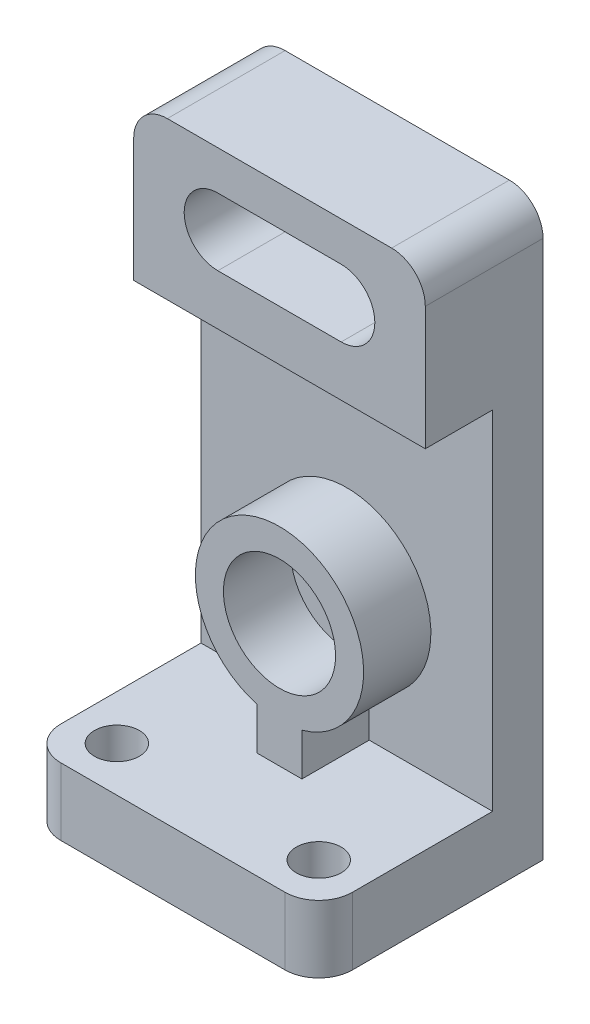
ISO-10303-21;
HEADER;
FILE_DESCRIPTION(('STEP AP214'),'2;1');
FILE_NAME('part.step','',(''),(''),'','','');
FILE_SCHEMA(('AUTOMOTIVE_DESIGN { 1 0 10303 214 1 1 1 1 }'));
ENDSEC;
DATA;
#1=APPLICATION_CONTEXT('core data for automotive mechanical design processes');
#2=APPLICATION_PROTOCOL_DEFINITION('international standard','automotive_design',2000,#1);
#3=PRODUCT_CONTEXT('',#1,'mechanical');
#4=PRODUCT('Part','Part','',(#3));
#5=PRODUCT_RELATED_PRODUCT_CATEGORY('part','',(#4));
#6=PRODUCT_DEFINITION_FORMATION('','',#4);
#7=PRODUCT_DEFINITION_CONTEXT('part definition',#1,'design');
#8=PRODUCT_DEFINITION('design','',#6,#7);
#9=PRODUCT_DEFINITION_SHAPE('','',#8);
#10=(LENGTH_UNIT() NAMED_UNIT(*) SI_UNIT(.MILLI.,.METRE.));
#11=(NAMED_UNIT(*) PLANE_ANGLE_UNIT() SI_UNIT($,.RADIAN.));
#12=(NAMED_UNIT(*) SI_UNIT($,.STERADIAN.) SOLID_ANGLE_UNIT());
#13=UNCERTAINTY_MEASURE_WITH_UNIT(LENGTH_MEASURE(1.E-05),#10,'distance_accuracy_value','');
#14=(GEOMETRIC_REPRESENTATION_CONTEXT(3) GLOBAL_UNCERTAINTY_ASSIGNED_CONTEXT((#13)) GLOBAL_UNIT_ASSIGNED_CONTEXT((#10,
#11,#12)) REPRESENTATION_CONTEXT('',''));
#15=CARTESIAN_POINT('',(0.,0.,0.));
#16=DIRECTION('',(0.,0.,1.));
#17=DIRECTION('',(1.,0.,0.));
#18=AXIS2_PLACEMENT_3D('',#15,#16,#17);
#19=CARTESIAN_POINT('',(46.,96.,9.));
#20=DIRECTION('',(0.,0.,1.));
#21=DIRECTION('',(1.,0.,0.));
#22=AXIS2_PLACEMENT_3D('',#19,#20,#21);
#23=PLANE('',#22);
#24=DIRECTION('',(1.,0.,0.));
#25=VECTOR('',#24,1.);
#26=CARTESIAN_POINT('',(46.,12.,9.));
#27=LINE('',#26,#25);
#28=CARTESIAN_POINT('',(0.,12.,9.));
#29=VERTEX_POINT('',#28);
#30=CARTESIAN_POINT('',(22.,12.,9.));
#31=VERTEX_POINT('',#30);
#32=EDGE_CURVE('E259',#29,#31,#27,.T.);
#33=ORIENTED_EDGE('',*,*,#32,.T.);
#34=DIRECTION('',(0.,-1.,0.));
#35=VECTOR('',#34,1.);
#36=CARTESIAN_POINT('',(22.,12.,9.));
#37=LINE('',#36,#35);
#38=CARTESIAN_POINT('',(22.,19.543167705199,9.));
#39=VERTEX_POINT('',#38);
#40=EDGE_CURVE('E392',#39,#31,#37,.T.);
#41=ORIENTED_EDGE('',*,*,#40,.F.);
#42=CARTESIAN_POINT('',(26.,34.,9.));
#43=DIRECTION('',(0.,0.,1.));
#44=DIRECTION('',(1.,0.,0.));
#45=AXIS2_PLACEMENT_3D('',#42,#43,#44);
#46=CIRCLE('',#45,15.);
#47=CARTESIAN_POINT('',(30.,19.543167705199,9.));
#48=VERTEX_POINT('',#47);
#49=EDGE_CURVE('E203',#48,#39,#46,.T.);
#50=ORIENTED_EDGE('',*,*,#49,.F.);
#51=DIRECTION('',(0.,1.,0.));
#52=VECTOR('',#51,1.);
#53=CARTESIAN_POINT('',(30.,19.543167705199,9.));
#54=LINE('',#53,#52);
#55=CARTESIAN_POINT('',(30.,12.,9.));
#56=VERTEX_POINT('',#55);
#57=EDGE_CURVE('E202',#56,#48,#54,.T.);
#58=ORIENTED_EDGE('',*,*,#57,.F.);
#59=CARTESIAN_POINT('',(52.,12.,9.));
#60=VERTEX_POINT('',#59);
#61=EDGE_CURVE('E252',#56,#60,#27,.T.);
#62=ORIENTED_EDGE('',*,*,#61,.T.);
#63=DIRECTION('',(0.,1.,0.));
#64=VECTOR('',#63,1.);
#65=CARTESIAN_POINT('',(52.,0.,9.));
#66=LINE('',#65,#64);
#67=CARTESIAN_POINT('',(52.,74.,9.));
#68=VERTEX_POINT('',#67);
#69=EDGE_CURVE('E319',#60,#68,#66,.T.);
#70=ORIENTED_EDGE('',*,*,#69,.T.);
#71=DIRECTION('',(-1.,0.,0.));
#72=VECTOR('',#71,1.);
#73=CARTESIAN_POINT('',(0.,74.,9.));
#74=LINE('',#73,#72);
#75=CARTESIAN_POINT('',(0.,74.,9.));
#76=VERTEX_POINT('',#75);
#77=EDGE_CURVE('E289',#68,#76,#74,.T.);
#78=ORIENTED_EDGE('',*,*,#77,.T.);
#79=DIRECTION('',(0.,-1.,0.));
#80=VECTOR('',#79,1.);
#81=CARTESIAN_POINT('',(0.,96.,9.));
#82=LINE('',#81,#80);
#83=EDGE_CURVE('E67',#76,#29,#82,.T.);
#84=ORIENTED_EDGE('',*,*,#83,.T.);
#85=EDGE_LOOP('',(#33,#41,#50,#58,#62,#70,#78,#84));
#86=FACE_BOUND('',#85,.T.);
#87=ADVANCED_FACE('F50',(#86),#23,.T.);
#88=CARTESIAN_POINT('',(46.,12.,34.));
#89=DIRECTION('',(0.,-1.,0.));
#90=DIRECTION('',(0.,0.,-1.));
#91=AXIS2_PLACEMENT_3D('',#88,#89,#90);
#92=PLANE('',#91);
#93=CARTESIAN_POINT('',(44.,12.,32.));
#94=DIRECTION('',(0.,1.,0.));
#95=DIRECTION('',(0.,0.,1.));
#96=AXIS2_PLACEMENT_3D('',#93,#94,#95);
#97=CIRCLE('',#96,4.);
#98=CARTESIAN_POINT('',(44.,12.,36.));
#99=VERTEX_POINT('',#98);
#100=EDGE_CURVE('E210',#99,#99,#97,.T.);
#101=ORIENTED_EDGE('',*,*,#100,.F.);
#102=EDGE_LOOP('',(#101));
#103=FACE_BOUND('',#102,.T.);
#104=CARTESIAN_POINT('',(8.,12.,32.));
#105=DIRECTION('',(0.,1.,0.));
#106=DIRECTION('',(0.,0.,1.));
#107=AXIS2_PLACEMENT_3D('',#104,#105,#106);
#108=CIRCLE('',#107,4.);
#109=CARTESIAN_POINT('',(8.,12.,36.));
#110=VERTEX_POINT('',#109);
#111=EDGE_CURVE('E217',#110,#110,#108,.T.);
#112=ORIENTED_EDGE('',*,*,#111,.F.);
#113=EDGE_LOOP('',(#112));
#114=FACE_BOUND('',#113,.T.);
#115=DIRECTION('',(0.,0.,-1.));
#116=VECTOR('',#115,1.);
#117=CARTESIAN_POINT('',(22.,12.,21.));
#118=LINE('',#117,#116);
#119=CARTESIAN_POINT('',(22.,12.,21.));
#120=VERTEX_POINT('',#119);
#121=EDGE_CURVE('E65',#120,#31,#118,.T.);
#122=ORIENTED_EDGE('',*,*,#121,.T.);
#123=ORIENTED_EDGE('',*,*,#32,.F.);
#124=DIRECTION('',(0.,0.,-1.));
#125=VECTOR('',#124,1.);
#126=CARTESIAN_POINT('',(0.,12.,9.));
#127=LINE('',#126,#125);
#128=CARTESIAN_POINT('',(0.,12.,34.));
#129=VERTEX_POINT('',#128);
#130=EDGE_CURVE('E223',#129,#29,#127,.T.);
#131=ORIENTED_EDGE('',*,*,#130,.F.);
#132=CARTESIAN_POINT('',(6.,12.,34.));
#133=DIRECTION('',(0.,-1.,0.));
#134=DIRECTION('',(0.,0.,-1.));
#135=AXIS2_PLACEMENT_3D('',#132,#133,#134);
#136=CIRCLE('',#135,6.);
#137=CARTESIAN_POINT('',(6.,12.,40.));
#138=VERTEX_POINT('',#137);
#139=EDGE_CURVE('E240',#138,#129,#136,.T.);
#140=ORIENTED_EDGE('',*,*,#139,.F.);
#141=DIRECTION('',(-1.,0.,0.));
#142=VECTOR('',#141,1.);
#143=CARTESIAN_POINT('',(6.,12.,40.));
#144=LINE('',#143,#142);
#145=CARTESIAN_POINT('',(46.,12.,40.));
#146=VERTEX_POINT('',#145);
#147=EDGE_CURVE('E234',#146,#138,#144,.T.);
#148=ORIENTED_EDGE('',*,*,#147,.F.);
#149=CARTESIAN_POINT('',(46.,12.,34.));
#150=DIRECTION('',(0.,-1.,0.));
#151=DIRECTION('',(0.,0.,-1.));
#152=AXIS2_PLACEMENT_3D('',#149,#150,#151);
#153=CIRCLE('',#152,6.);
#154=CARTESIAN_POINT('',(52.,12.,34.));
#155=VERTEX_POINT('',#154);
#156=EDGE_CURVE('E233',#155,#146,#153,.T.);
#157=ORIENTED_EDGE('',*,*,#156,.F.);
#158=DIRECTION('',(0.,0.,1.));
#159=VECTOR('',#158,1.);
#160=CARTESIAN_POINT('',(52.,12.,0.));
#161=LINE('',#160,#159);
#162=EDGE_CURVE('E226',#60,#155,#161,.T.);
#163=ORIENTED_EDGE('',*,*,#162,.F.);
#164=ORIENTED_EDGE('',*,*,#61,.F.);
#165=DIRECTION('',(0.,0.,-1.));
#166=VECTOR('',#165,1.);
#167=CARTESIAN_POINT('',(30.,12.,21.));
#168=LINE('',#167,#166);
#169=CARTESIAN_POINT('',(30.,12.,21.));
#170=VERTEX_POINT('',#169);
#171=EDGE_CURVE('E215',#170,#56,#168,.T.);
#172=ORIENTED_EDGE('',*,*,#171,.F.);
#173=DIRECTION('',(1.,0.,0.));
#174=VECTOR('',#173,1.);
#175=CARTESIAN_POINT('',(30.,12.,21.));
#176=LINE('',#175,#174);
#177=EDGE_CURVE('E192',#120,#170,#176,.T.);
#178=ORIENTED_EDGE('',*,*,#177,.F.);
#179=EDGE_LOOP('',(#122,#123,#131,#140,#148,#157,#163,#164,#172,#178));
#180=FACE_BOUND('',#179,.T.);
#181=ADVANCED_FACE('F382',(#103,#114,#180),#92,.F.);
#182=CARTESIAN_POINT('',(0.,96.,9.));
#183=DIRECTION('',(1.,0.,0.));
#184=DIRECTION('',(0.,0.,-1.));
#185=AXIS2_PLACEMENT_3D('',#182,#183,#184);
#186=PLANE('',#185);
#187=DIRECTION('',(0.,0.,-1.));
#188=VECTOR('',#187,1.);
#189=CARTESIAN_POINT('',(0.,0.,9.));
#190=LINE('',#189,#188);
#191=CARTESIAN_POINT('',(0.,0.,34.));
#192=VERTEX_POINT('',#191);
#193=CARTESIAN_POINT('',(0.,0.,0.));
#194=VERTEX_POINT('',#193);
#195=EDGE_CURVE('E11',#192,#194,#190,.T.);
#196=ORIENTED_EDGE('',*,*,#195,.F.);
#197=DIRECTION('',(0.,-1.,0.));
#198=VECTOR('',#197,1.);
#199=CARTESIAN_POINT('',(0.,12.,34.));
#200=LINE('',#199,#198);
#201=EDGE_CURVE('E247',#129,#192,#200,.T.);
#202=ORIENTED_EDGE('',*,*,#201,.F.);
#203=ORIENTED_EDGE('',*,*,#130,.T.);
#204=ORIENTED_EDGE('',*,*,#83,.F.);
#205=DIRECTION('',(0.,0.,-1.));
#206=VECTOR('',#205,1.);
#207=CARTESIAN_POINT('',(0.,74.,21.));
#208=LINE('',#207,#206);
#209=CARTESIAN_POINT('',(0.,74.,21.));
#210=VERTEX_POINT('',#209);
#211=EDGE_CURVE('E309',#210,#76,#208,.T.);
#212=ORIENTED_EDGE('',*,*,#211,.F.);
#213=DIRECTION('',(0.,-1.,0.));
#214=VECTOR('',#213,1.);
#215=CARTESIAN_POINT('',(0.,0.,21.));
#216=LINE('',#215,#214);
#217=CARTESIAN_POINT('',(0.,96.,21.));
#218=VERTEX_POINT('',#217);
#219=EDGE_CURVE('E308',#218,#210,#216,.T.);
#220=ORIENTED_EDGE('',*,*,#219,.F.);
#221=DIRECTION('',(0.,0.,-1.));
#222=VECTOR('',#221,1.);
#223=CARTESIAN_POINT('',(0.,96.,9.));
#224=LINE('',#223,#222);
#225=CARTESIAN_POINT('',(0.,96.,0.));
#226=VERTEX_POINT('',#225);
#227=EDGE_CURVE('E322',#218,#226,#224,.T.);
#228=ORIENTED_EDGE('',*,*,#227,.T.);
#229=DIRECTION('',(0.,-1.,0.));
#230=VECTOR('',#229,1.);
#231=CARTESIAN_POINT('',(0.,96.,0.));
#232=LINE('',#231,#230);
#233=EDGE_CURVE('E317',#226,#194,#232,.T.);
#234=ORIENTED_EDGE('',*,*,#233,.T.);
#235=EDGE_LOOP('',(#196,#202,#203,#204,#212,#220,#228,#234));
#236=FACE_BOUND('',#235,.T.);
#237=ADVANCED_FACE('F47',(#236),#186,.F.);
#238=CARTESIAN_POINT('',(0.,0.,9.));
#239=DIRECTION('',(0.,1.,0.));
#240=DIRECTION('',(0.,0.,1.));
#241=AXIS2_PLACEMENT_3D('',#238,#239,#240);
#242=PLANE('',#241);
#243=CARTESIAN_POINT('',(8.,0.,32.));
#244=DIRECTION('',(0.,1.,0.));
#245=DIRECTION('',(0.,0.,1.));
#246=AXIS2_PLACEMENT_3D('',#243,#244,#245);
#247=CIRCLE('',#246,4.);
#248=CARTESIAN_POINT('',(8.,0.,36.));
#249=VERTEX_POINT('',#248);
#250=EDGE_CURVE('E218',#249,#249,#247,.T.);
#251=ORIENTED_EDGE('',*,*,#250,.T.);
#252=EDGE_LOOP('',(#251));
#253=FACE_BOUND('',#252,.T.);
#254=CARTESIAN_POINT('',(44.,0.,32.));
#255=DIRECTION('',(0.,1.,0.));
#256=DIRECTION('',(0.,0.,1.));
#257=AXIS2_PLACEMENT_3D('',#254,#255,#256);
#258=CIRCLE('',#257,4.);
#259=CARTESIAN_POINT('',(44.,0.,36.));
#260=VERTEX_POINT('',#259);
#261=EDGE_CURVE('E208',#260,#260,#258,.T.);
#262=ORIENTED_EDGE('',*,*,#261,.T.);
#263=EDGE_LOOP('',(#262));
#264=FACE_BOUND('',#263,.T.);
#265=DIRECTION('',(1.,0.,0.));
#266=VECTOR('',#265,1.);
#267=CARTESIAN_POINT('',(0.,0.,0.));
#268=LINE('',#267,#266);
#269=CARTESIAN_POINT('',(52.,0.,0.));
#270=VERTEX_POINT('',#269);
#271=EDGE_CURVE('E324',#194,#270,#268,.T.);
#272=ORIENTED_EDGE('',*,*,#271,.T.);
#273=DIRECTION('',(0.,0.,-1.));
#274=VECTOR('',#273,1.);
#275=CARTESIAN_POINT('',(52.,0.,9.));
#276=LINE('',#275,#274);
#277=CARTESIAN_POINT('',(52.,0.,34.));
#278=VERTEX_POINT('',#277);
#279=EDGE_CURVE('E54',#278,#270,#276,.T.);
#280=ORIENTED_EDGE('',*,*,#279,.F.);
#281=CARTESIAN_POINT('',(46.,0.,34.));
#282=DIRECTION('',(0.,-1.,0.));
#283=DIRECTION('',(0.,0.,-1.));
#284=AXIS2_PLACEMENT_3D('',#281,#282,#283);
#285=CIRCLE('',#284,6.);
#286=CARTESIAN_POINT('',(46.,0.,40.));
#287=VERTEX_POINT('',#286);
#288=EDGE_CURVE('E219',#278,#287,#285,.T.);
#289=ORIENTED_EDGE('',*,*,#288,.T.);
#290=DIRECTION('',(-1.,0.,0.));
#291=VECTOR('',#290,1.);
#292=CARTESIAN_POINT('',(6.,0.,40.));
#293=LINE('',#292,#291);
#294=CARTESIAN_POINT('',(6.,0.,40.));
#295=VERTEX_POINT('',#294);
#296=EDGE_CURVE('E243',#287,#295,#293,.T.);
#297=ORIENTED_EDGE('',*,*,#296,.T.);
#298=CARTESIAN_POINT('',(6.,0.,34.));
#299=DIRECTION('',(0.,-1.,0.));
#300=DIRECTION('',(0.,0.,-1.));
#301=AXIS2_PLACEMENT_3D('',#298,#299,#300);
#302=CIRCLE('',#301,6.);
#303=EDGE_CURVE('E230',#295,#192,#302,.T.);
#304=ORIENTED_EDGE('',*,*,#303,.T.);
#305=ORIENTED_EDGE('',*,*,#195,.T.);
#306=EDGE_LOOP('',(#272,#280,#289,#297,#304,#305));
#307=FACE_BOUND('',#306,.T.);
#308=ADVANCED_FACE('F389',(#253,#264,#307),#242,.F.);
#309=CARTESIAN_POINT('',(52.,0.,9.));
#310=DIRECTION('',(-1.,0.,0.));
#311=DIRECTION('',(0.,0.,1.));
#312=AXIS2_PLACEMENT_3D('',#309,#310,#311);
#313=PLANE('',#312);
#314=DIRECTION('',(0.,1.,0.));
#315=VECTOR('',#314,1.);
#316=CARTESIAN_POINT('',(52.,0.,0.));
#317=LINE('',#316,#315);
#318=CARTESIAN_POINT('',(52.,96.,0.));
#319=VERTEX_POINT('',#318);
#320=EDGE_CURVE('E323',#270,#319,#317,.T.);
#321=ORIENTED_EDGE('',*,*,#320,.T.);
#322=DIRECTION('',(0.,0.,-1.));
#323=VECTOR('',#322,1.);
#324=CARTESIAN_POINT('',(52.,96.,9.));
#325=LINE('',#324,#323);
#326=CARTESIAN_POINT('',(52.,96.,21.));
#327=VERTEX_POINT('',#326);
#328=EDGE_CURVE('E338',#327,#319,#325,.T.);
#329=ORIENTED_EDGE('',*,*,#328,.F.);
#330=DIRECTION('',(0.,1.,0.));
#331=VECTOR('',#330,1.);
#332=CARTESIAN_POINT('',(52.,0.,21.));
#333=LINE('',#332,#331);
#334=CARTESIAN_POINT('',(52.,74.,21.));
#335=VERTEX_POINT('',#334);
#336=EDGE_CURVE('E298',#335,#327,#333,.T.);
#337=ORIENTED_EDGE('',*,*,#336,.F.);
#338=DIRECTION('',(0.,0.,-1.));
#339=VECTOR('',#338,1.);
#340=CARTESIAN_POINT('',(52.,74.,21.));
#341=LINE('',#340,#339);
#342=EDGE_CURVE('E312',#335,#68,#341,.T.);
#343=ORIENTED_EDGE('',*,*,#342,.T.);
#344=ORIENTED_EDGE('',*,*,#69,.F.);
#345=ORIENTED_EDGE('',*,*,#162,.T.);
#346=DIRECTION('',(0.,-1.,0.));
#347=VECTOR('',#346,1.);
#348=CARTESIAN_POINT('',(52.,12.,34.));
#349=LINE('',#348,#347);
#350=EDGE_CURVE('E239',#155,#278,#349,.T.);
#351=ORIENTED_EDGE('',*,*,#350,.T.);
#352=ORIENTED_EDGE('',*,*,#279,.T.);
#353=EDGE_LOOP('',(#321,#329,#337,#343,#344,#345,#351,#352));
#354=FACE_BOUND('',#353,.T.);
#355=ADVANCED_FACE('F343',(#354),#313,.F.);
#356=CARTESIAN_POINT('',(46.,96.,9.));
#357=DIRECTION('',(0.,0.,-1.));
#358=DIRECTION('',(-1.,0.,0.));
#359=AXIS2_PLACEMENT_3D('',#356,#357,#358);
#360=CYLINDRICAL_SURFACE('',#359,6.);
#361=CARTESIAN_POINT('',(46.,96.,0.));
#362=DIRECTION('',(0.,0.,1.));
#363=DIRECTION('',(1.,0.,0.));
#364=AXIS2_PLACEMENT_3D('',#361,#362,#363);
#365=CIRCLE('',#364,6.);
#366=CARTESIAN_POINT('',(46.,102.,0.));
#367=VERTEX_POINT('',#366);
#368=EDGE_CURVE('E330',#319,#367,#365,.T.);
#369=ORIENTED_EDGE('',*,*,#368,.T.);
#370=DIRECTION('',(0.,0.,-1.));
#371=VECTOR('',#370,1.);
#372=CARTESIAN_POINT('',(46.,102.,9.));
#373=LINE('',#372,#371);
#374=CARTESIAN_POINT('',(46.,102.,21.));
#375=VERTEX_POINT('',#374);
#376=EDGE_CURVE('E340',#375,#367,#373,.T.);
#377=ORIENTED_EDGE('',*,*,#376,.F.);
#378=CARTESIAN_POINT('',(46.,96.,21.));
#379=DIRECTION('',(0.,0.,1.));
#380=DIRECTION('',(1.,0.,0.));
#381=AXIS2_PLACEMENT_3D('',#378,#379,#380);
#382=CIRCLE('',#381,6.);
#383=EDGE_CURVE('E299',#327,#375,#382,.T.);
#384=ORIENTED_EDGE('',*,*,#383,.F.);
#385=ORIENTED_EDGE('',*,*,#328,.T.);
#386=EDGE_LOOP('',(#369,#377,#384,#385));
#387=FACE_BOUND('',#386,.T.);
#388=ADVANCED_FACE('F356',(#387),#360,.T.);
#389=CARTESIAN_POINT('',(46.,102.,9.));
#390=DIRECTION('',(0.,-1.,0.));
#391=DIRECTION('',(0.,0.,-1.));
#392=AXIS2_PLACEMENT_3D('',#389,#390,#391);
#393=PLANE('',#392);
#394=DIRECTION('',(-1.,0.,0.));
#395=VECTOR('',#394,1.);
#396=CARTESIAN_POINT('',(46.,102.,0.));
#397=LINE('',#396,#395);
#398=CARTESIAN_POINT('',(6.,102.,0.));
#399=VERTEX_POINT('',#398);
#400=EDGE_CURVE('E329',#367,#399,#397,.T.);
#401=ORIENTED_EDGE('',*,*,#400,.T.);
#402=DIRECTION('',(0.,0.,-1.));
#403=VECTOR('',#402,1.);
#404=CARTESIAN_POINT('',(6.,102.,9.));
#405=LINE('',#404,#403);
#406=CARTESIAN_POINT('',(6.,102.,21.));
#407=VERTEX_POINT('',#406);
#408=EDGE_CURVE('E331',#407,#399,#405,.T.);
#409=ORIENTED_EDGE('',*,*,#408,.F.);
#410=DIRECTION('',(-1.,0.,0.));
#411=VECTOR('',#410,1.);
#412=CARTESIAN_POINT('',(0.,102.,21.));
#413=LINE('',#412,#411);
#414=EDGE_CURVE('E305',#375,#407,#413,.T.);
#415=ORIENTED_EDGE('',*,*,#414,.F.);
#416=ORIENTED_EDGE('',*,*,#376,.T.);
#417=EDGE_LOOP('',(#401,#409,#415,#416));
#418=FACE_BOUND('',#417,.T.);
#419=ADVANCED_FACE('F365',(#418),#393,.F.);
#420=CARTESIAN_POINT('',(6.,96.,9.));
#421=DIRECTION('',(0.,0.,-1.));
#422=DIRECTION('',(-1.,0.,0.));
#423=AXIS2_PLACEMENT_3D('',#420,#421,#422);
#424=CYLINDRICAL_SURFACE('',#423,6.);
#425=CARTESIAN_POINT('',(6.,96.,0.));
#426=DIRECTION('',(0.,0.,1.));
#427=DIRECTION('',(1.,0.,0.));
#428=AXIS2_PLACEMENT_3D('',#425,#426,#427);
#429=CIRCLE('',#428,6.);
#430=EDGE_CURVE('E316',#399,#226,#429,.T.);
#431=ORIENTED_EDGE('',*,*,#430,.T.);
#432=ORIENTED_EDGE('',*,*,#227,.F.);
#433=CARTESIAN_POINT('',(6.,96.,21.));
#434=DIRECTION('',(0.,0.,1.));
#435=DIRECTION('',(1.,0.,0.));
#436=AXIS2_PLACEMENT_3D('',#433,#434,#435);
#437=CIRCLE('',#436,6.);
#438=EDGE_CURVE('E304',#407,#218,#437,.T.);
#439=ORIENTED_EDGE('',*,*,#438,.F.);
#440=ORIENTED_EDGE('',*,*,#408,.T.);
#441=EDGE_LOOP('',(#431,#432,#439,#440));
#442=FACE_BOUND('',#441,.T.);
#443=ADVANCED_FACE('F367',(#442),#424,.T.);
#444=CARTESIAN_POINT('',(46.,96.,0.));
#445=DIRECTION('',(0.,0.,1.));
#446=DIRECTION('',(1.,0.,0.));
#447=AXIS2_PLACEMENT_3D('',#444,#445,#446);
#448=PLANE('',#447);
#449=ORIENTED_EDGE('',*,*,#271,.F.);
#450=ORIENTED_EDGE('',*,*,#233,.F.);
#451=ORIENTED_EDGE('',*,*,#430,.F.);
#452=ORIENTED_EDGE('',*,*,#400,.F.);
#453=ORIENTED_EDGE('',*,*,#368,.F.);
#454=ORIENTED_EDGE('',*,*,#320,.F.);
#455=EDGE_LOOP('',(#449,#450,#451,#452,#453,#454));
#456=FACE_BOUND('',#455,.T.);
#457=DIRECTION('',(1.,0.,0.));
#458=VECTOR('',#457,1.);
#459=CARTESIAN_POINT('',(15.,83.,0.));
#460=LINE('',#459,#458);
#461=CARTESIAN_POINT('',(15.,83.,0.));
#462=VERTEX_POINT('',#461);
#463=CARTESIAN_POINT('',(37.,83.,0.));
#464=VERTEX_POINT('',#463);
#465=EDGE_CURVE('E270',#462,#464,#460,.T.);
#466=ORIENTED_EDGE('',*,*,#465,.T.);
#467=CARTESIAN_POINT('',(37.,89.,0.));
#468=DIRECTION('',(0.,0.,1.));
#469=DIRECTION('',(1.,0.,0.));
#470=AXIS2_PLACEMENT_3D('',#467,#468,#469);
#471=CIRCLE('',#470,6.);
#472=CARTESIAN_POINT('',(37.,95.,0.));
#473=VERTEX_POINT('',#472);
#474=EDGE_CURVE('E272',#464,#473,#471,.T.);
#475=ORIENTED_EDGE('',*,*,#474,.T.);
#476=DIRECTION('',(-1.,0.,0.));
#477=VECTOR('',#476,1.);
#478=CARTESIAN_POINT('',(37.,95.,0.));
#479=LINE('',#478,#477);
#480=CARTESIAN_POINT('',(15.,95.,0.));
#481=VERTEX_POINT('',#480);
#482=EDGE_CURVE('E263',#473,#481,#479,.T.);
#483=ORIENTED_EDGE('',*,*,#482,.T.);
#484=CARTESIAN_POINT('',(15.,89.,0.));
#485=DIRECTION('',(0.,0.,1.));
#486=DIRECTION('',(1.,0.,0.));
#487=AXIS2_PLACEMENT_3D('',#484,#485,#486);
#488=CIRCLE('',#487,6.);
#489=EDGE_CURVE('E264',#481,#462,#488,.T.);
#490=ORIENTED_EDGE('',*,*,#489,.T.);
#491=EDGE_LOOP('',(#466,#475,#483,#490));
#492=FACE_BOUND('',#491,.T.);
#493=ADVANCED_FACE('F354',(#456,#492),#448,.F.);
#494=CARTESIAN_POINT('',(0.,74.,21.));
#495=DIRECTION('',(0.,-1.,0.));
#496=DIRECTION('',(0.,0.,-1.));
#497=AXIS2_PLACEMENT_3D('',#494,#495,#496);
#498=PLANE('',#497);
#499=ORIENTED_EDGE('',*,*,#77,.F.);
#500=ORIENTED_EDGE('',*,*,#342,.F.);
#501=DIRECTION('',(-1.,0.,0.));
#502=VECTOR('',#501,1.);
#503=CARTESIAN_POINT('',(0.,74.,21.));
#504=LINE('',#503,#502);
#505=EDGE_CURVE('E291',#335,#210,#504,.T.);
#506=ORIENTED_EDGE('',*,*,#505,.T.);
#507=ORIENTED_EDGE('',*,*,#211,.T.);
#508=EDGE_LOOP('',(#499,#500,#506,#507));
#509=FACE_BOUND('',#508,.T.);
#510=ADVANCED_FACE('F374',(#509),#498,.T.);
#511=CARTESIAN_POINT('',(0.,0.,21.));
#512=DIRECTION('',(0.,0.,1.));
#513=DIRECTION('',(1.,0.,0.));
#514=AXIS2_PLACEMENT_3D('',#511,#512,#513);
#515=PLANE('',#514);
#516=CARTESIAN_POINT('',(37.,89.,21.));
#517=DIRECTION('',(0.,0.,1.));
#518=DIRECTION('',(1.,0.,0.));
#519=AXIS2_PLACEMENT_3D('',#516,#517,#518);
#520=CIRCLE('',#519,6.);
#521=CARTESIAN_POINT('',(37.,83.,21.));
#522=VERTEX_POINT('',#521);
#523=CARTESIAN_POINT('',(37.,95.,21.));
#524=VERTEX_POINT('',#523);
#525=EDGE_CURVE('E262',#522,#524,#520,.T.);
#526=ORIENTED_EDGE('',*,*,#525,.F.);
#527=DIRECTION('',(1.,0.,0.));
#528=VECTOR('',#527,1.);
#529=CARTESIAN_POINT('',(15.,83.,21.));
#530=LINE('',#529,#528);
#531=CARTESIAN_POINT('',(15.,83.,21.));
#532=VERTEX_POINT('',#531);
#533=EDGE_CURVE('E278',#532,#522,#530,.T.);
#534=ORIENTED_EDGE('',*,*,#533,.F.);
#535=CARTESIAN_POINT('',(15.,89.,21.));
#536=DIRECTION('',(0.,0.,1.));
#537=DIRECTION('',(1.,0.,0.));
#538=AXIS2_PLACEMENT_3D('',#535,#536,#537);
#539=CIRCLE('',#538,6.);
#540=CARTESIAN_POINT('',(15.,95.,21.));
#541=VERTEX_POINT('',#540);
#542=EDGE_CURVE('E280',#541,#532,#539,.T.);
#543=ORIENTED_EDGE('',*,*,#542,.F.);
#544=DIRECTION('',(-1.,0.,0.));
#545=VECTOR('',#544,1.);
#546=CARTESIAN_POINT('',(26.,95.,21.));
#547=LINE('',#546,#545);
#548=EDGE_CURVE('E258',#524,#541,#547,.T.);
#549=ORIENTED_EDGE('',*,*,#548,.F.);
#550=EDGE_LOOP('',(#526,#534,#543,#549));
#551=FACE_BOUND('',#550,.T.);
#552=ORIENTED_EDGE('',*,*,#505,.F.);
#553=ORIENTED_EDGE('',*,*,#336,.T.);
#554=ORIENTED_EDGE('',*,*,#383,.T.);
#555=ORIENTED_EDGE('',*,*,#414,.T.);
#556=ORIENTED_EDGE('',*,*,#438,.T.);
#557=ORIENTED_EDGE('',*,*,#219,.T.);
#558=EDGE_LOOP('',(#552,#553,#554,#555,#556,#557));
#559=FACE_BOUND('',#558,.T.);
#560=ADVANCED_FACE('F366',(#551,#559),#515,.T.);
#561=CARTESIAN_POINT('',(37.,89.,0.));
#562=DIRECTION('',(0.,0.,1.));
#563=DIRECTION('',(1.,0.,0.));
#564=AXIS2_PLACEMENT_3D('',#561,#562,#563);
#565=CYLINDRICAL_SURFACE('',#564,6.);
#566=ORIENTED_EDGE('',*,*,#525,.T.);
#567=DIRECTION('',(0.,0.,1.));
#568=VECTOR('',#567,1.);
#569=CARTESIAN_POINT('',(37.,95.,0.));
#570=LINE('',#569,#568);
#571=EDGE_CURVE('E284',#473,#524,#570,.T.);
#572=ORIENTED_EDGE('',*,*,#571,.F.);
#573=ORIENTED_EDGE('',*,*,#474,.F.);
#574=DIRECTION('',(0.,0.,1.));
#575=VECTOR('',#574,1.);
#576=CARTESIAN_POINT('',(37.,83.,0.));
#577=LINE('',#576,#575);
#578=EDGE_CURVE('E290',#464,#522,#577,.T.);
#579=ORIENTED_EDGE('',*,*,#578,.T.);
#580=EDGE_LOOP('',(#566,#572,#573,#579));
#581=FACE_BOUND('',#580,.T.);
#582=ADVANCED_FACE('F481',(#581),#565,.F.);
#583=CARTESIAN_POINT('',(15.,83.,0.));
#584=DIRECTION('',(0.,-1.,0.));
#585=DIRECTION('',(0.,0.,-1.));
#586=AXIS2_PLACEMENT_3D('',#583,#584,#585);
#587=PLANE('',#586);
#588=ORIENTED_EDGE('',*,*,#533,.T.);
#589=ORIENTED_EDGE('',*,*,#578,.F.);
#590=ORIENTED_EDGE('',*,*,#465,.F.);
#591=DIRECTION('',(0.,0.,1.));
#592=VECTOR('',#591,1.);
#593=CARTESIAN_POINT('',(15.,83.,0.));
#594=LINE('',#593,#592);
#595=EDGE_CURVE('E288',#462,#532,#594,.T.);
#596=ORIENTED_EDGE('',*,*,#595,.T.);
#597=EDGE_LOOP('',(#588,#589,#590,#596));
#598=FACE_BOUND('',#597,.T.);
#599=ADVANCED_FACE('F487',(#598),#587,.F.);
#600=CARTESIAN_POINT('',(15.,89.,0.));
#601=DIRECTION('',(0.,0.,1.));
#602=DIRECTION('',(1.,0.,0.));
#603=AXIS2_PLACEMENT_3D('',#600,#601,#602);
#604=CYLINDRICAL_SURFACE('',#603,6.);
#605=ORIENTED_EDGE('',*,*,#542,.T.);
#606=ORIENTED_EDGE('',*,*,#595,.F.);
#607=ORIENTED_EDGE('',*,*,#489,.F.);
#608=DIRECTION('',(0.,0.,1.));
#609=VECTOR('',#608,1.);
#610=CARTESIAN_POINT('',(15.,95.,0.));
#611=LINE('',#610,#609);
#612=EDGE_CURVE('E274',#481,#541,#611,.T.);
#613=ORIENTED_EDGE('',*,*,#612,.T.);
#614=EDGE_LOOP('',(#605,#606,#607,#613));
#615=FACE_BOUND('',#614,.T.);
#616=ADVANCED_FACE('F493',(#615),#604,.F.);
#617=CARTESIAN_POINT('',(26.,95.,0.));
#618=DIRECTION('',(0.,1.,0.));
#619=DIRECTION('',(0.,0.,1.));
#620=AXIS2_PLACEMENT_3D('',#617,#618,#619);
#621=PLANE('',#620);
#622=ORIENTED_EDGE('',*,*,#548,.T.);
#623=ORIENTED_EDGE('',*,*,#612,.F.);
#624=ORIENTED_EDGE('',*,*,#482,.F.);
#625=ORIENTED_EDGE('',*,*,#571,.T.);
#626=EDGE_LOOP('',(#622,#623,#624,#625));
#627=FACE_BOUND('',#626,.T.);
#628=ADVANCED_FACE('F479',(#627),#621,.F.);
#629=CARTESIAN_POINT('',(6.,12.,34.));
#630=DIRECTION('',(0.,-1.,0.));
#631=DIRECTION('',(0.,0.,-1.));
#632=AXIS2_PLACEMENT_3D('',#629,#630,#631);
#633=CYLINDRICAL_SURFACE('',#632,6.);
#634=ORIENTED_EDGE('',*,*,#303,.F.);
#635=DIRECTION('',(0.,-1.,0.));
#636=VECTOR('',#635,1.);
#637=CARTESIAN_POINT('',(6.,12.,40.));
#638=LINE('',#637,#636);
#639=EDGE_CURVE('E255',#138,#295,#638,.T.);
#640=ORIENTED_EDGE('',*,*,#639,.F.);
#641=ORIENTED_EDGE('',*,*,#139,.T.);
#642=ORIENTED_EDGE('',*,*,#201,.T.);
#643=EDGE_LOOP('',(#634,#640,#641,#642));
#644=FACE_BOUND('',#643,.T.);
#645=ADVANCED_FACE('F391',(#644),#633,.T.);
#646=CARTESIAN_POINT('',(6.,12.,40.));
#647=DIRECTION('',(0.,0.,1.));
#648=DIRECTION('',(1.,0.,0.));
#649=AXIS2_PLACEMENT_3D('',#646,#647,#648);
#650=PLANE('',#649);
#651=ORIENTED_EDGE('',*,*,#296,.F.);
#652=DIRECTION('',(0.,-1.,0.));
#653=VECTOR('',#652,1.);
#654=CARTESIAN_POINT('',(46.,12.,40.));
#655=LINE('',#654,#653);
#656=EDGE_CURVE('E251',#146,#287,#655,.T.);
#657=ORIENTED_EDGE('',*,*,#656,.F.);
#658=ORIENTED_EDGE('',*,*,#147,.T.);
#659=ORIENTED_EDGE('',*,*,#639,.T.);
#660=EDGE_LOOP('',(#651,#657,#658,#659));
#661=FACE_BOUND('',#660,.T.);
#662=ADVANCED_FACE('F393',(#661),#650,.T.);
#663=CARTESIAN_POINT('',(46.,12.,34.));
#664=DIRECTION('',(0.,-1.,0.));
#665=DIRECTION('',(0.,0.,-1.));
#666=AXIS2_PLACEMENT_3D('',#663,#664,#665);
#667=CYLINDRICAL_SURFACE('',#666,6.);
#668=ORIENTED_EDGE('',*,*,#288,.F.);
#669=ORIENTED_EDGE('',*,*,#350,.F.);
#670=ORIENTED_EDGE('',*,*,#156,.T.);
#671=ORIENTED_EDGE('',*,*,#656,.T.);
#672=EDGE_LOOP('',(#668,#669,#670,#671));
#673=FACE_BOUND('',#672,.T.);
#674=ADVANCED_FACE('F387',(#673),#667,.T.);
#675=CARTESIAN_POINT('',(44.,0.,32.));
#676=DIRECTION('',(0.,1.,0.));
#677=DIRECTION('',(0.,0.,1.));
#678=AXIS2_PLACEMENT_3D('',#675,#676,#677);
#679=CYLINDRICAL_SURFACE('',#678,4.);
#680=ORIENTED_EDGE('',*,*,#261,.F.);
#681=EDGE_LOOP('',(#680));
#682=FACE_BOUND('',#681,.T.);
#683=ORIENTED_EDGE('',*,*,#100,.T.);
#684=EDGE_LOOP('',(#683));
#685=FACE_BOUND('',#684,.T.);
#686=ADVANCED_FACE('F459',(#682,#685),#679,.F.);
#687=CARTESIAN_POINT('',(8.,0.,32.));
#688=DIRECTION('',(0.,1.,0.));
#689=DIRECTION('',(0.,0.,1.));
#690=AXIS2_PLACEMENT_3D('',#687,#688,#689);
#691=CYLINDRICAL_SURFACE('',#690,4.);
#692=ORIENTED_EDGE('',*,*,#250,.F.);
#693=EDGE_LOOP('',(#692));
#694=FACE_BOUND('',#693,.T.);
#695=ORIENTED_EDGE('',*,*,#111,.T.);
#696=EDGE_LOOP('',(#695));
#697=FACE_BOUND('',#696,.T.);
#698=ADVANCED_FACE('F464',(#694,#697),#691,.F.);
#699=CARTESIAN_POINT('',(26.,34.,21.));
#700=DIRECTION('',(0.,0.,-1.));
#701=DIRECTION('',(-1.,0.,0.));
#702=AXIS2_PLACEMENT_3D('',#699,#700,#701);
#703=CYLINDRICAL_SURFACE('',#702,15.);
#704=ORIENTED_EDGE('',*,*,#49,.T.);
#705=DIRECTION('',(0.,0.,-1.));
#706=VECTOR('',#705,1.);
#707=CARTESIAN_POINT('',(22.,19.543167705199,21.));
#708=LINE('',#707,#706);
#709=CARTESIAN_POINT('',(22.,19.543167705199,21.));
#710=VERTEX_POINT('',#709);
#711=EDGE_CURVE('E190',#710,#39,#708,.T.);
#712=ORIENTED_EDGE('',*,*,#711,.F.);
#713=CARTESIAN_POINT('',(26.,34.,21.));
#714=DIRECTION('',(0.,0.,1.));
#715=DIRECTION('',(1.,0.,0.));
#716=AXIS2_PLACEMENT_3D('',#713,#714,#715);
#717=CIRCLE('',#716,15.);
#718=CARTESIAN_POINT('',(30.,19.543167705199,21.));
#719=VERTEX_POINT('',#718);
#720=EDGE_CURVE('E195',#719,#710,#717,.T.);
#721=ORIENTED_EDGE('',*,*,#720,.F.);
#722=DIRECTION('',(0.,0.,-1.));
#723=VECTOR('',#722,1.);
#724=CARTESIAN_POINT('',(30.,19.543167705199,21.));
#725=LINE('',#724,#723);
#726=EDGE_CURVE('E401',#719,#48,#725,.T.);
#727=ORIENTED_EDGE('',*,*,#726,.T.);
#728=EDGE_LOOP('',(#704,#712,#721,#727));
#729=FACE_BOUND('',#728,.T.);
#730=ADVANCED_FACE('F205',(#729),#703,.T.);
#731=CARTESIAN_POINT('',(22.,12.,21.));
#732=DIRECTION('',(1.,0.,0.));
#733=DIRECTION('',(0.,0.,-1.));
#734=AXIS2_PLACEMENT_3D('',#731,#732,#733);
#735=PLANE('',#734);
#736=ORIENTED_EDGE('',*,*,#40,.T.);
#737=ORIENTED_EDGE('',*,*,#121,.F.);
#738=DIRECTION('',(0.,-1.,0.));
#739=VECTOR('',#738,1.);
#740=CARTESIAN_POINT('',(22.,12.,21.));
#741=LINE('',#740,#739);
#742=EDGE_CURVE('E182',#710,#120,#741,.T.);
#743=ORIENTED_EDGE('',*,*,#742,.F.);
#744=ORIENTED_EDGE('',*,*,#711,.T.);
#745=EDGE_LOOP('',(#736,#737,#743,#744));
#746=FACE_BOUND('',#745,.T.);
#747=ADVANCED_FACE('F184',(#746),#735,.F.);
#748=CARTESIAN_POINT('',(30.,19.543167705199,21.));
#749=DIRECTION('',(-1.,0.,0.));
#750=DIRECTION('',(0.,0.,1.));
#751=AXIS2_PLACEMENT_3D('',#748,#749,#750);
#752=PLANE('',#751);
#753=ORIENTED_EDGE('',*,*,#57,.T.);
#754=ORIENTED_EDGE('',*,*,#726,.F.);
#755=DIRECTION('',(0.,1.,0.));
#756=VECTOR('',#755,1.);
#757=CARTESIAN_POINT('',(30.,19.,21.));
#758=LINE('',#757,#756);
#759=EDGE_CURVE('E200',#170,#719,#758,.T.);
#760=ORIENTED_EDGE('',*,*,#759,.F.);
#761=ORIENTED_EDGE('',*,*,#171,.T.);
#762=EDGE_LOOP('',(#753,#754,#760,#761));
#763=FACE_BOUND('',#762,.T.);
#764=ADVANCED_FACE('F403',(#763),#752,.F.);
#765=CARTESIAN_POINT('',(26.,34.,21.));
#766=DIRECTION('',(0.,0.,1.));
#767=DIRECTION('',(1.,0.,0.));
#768=AXIS2_PLACEMENT_3D('',#765,#766,#767);
#769=PLANE('',#768);
#770=CARTESIAN_POINT('',(26.,34.,21.));
#771=DIRECTION('',(0.,0.,1.));
#772=DIRECTION('',(1.,0.,0.));
#773=AXIS2_PLACEMENT_3D('',#770,#771,#772);
#774=CIRCLE('',#773,10.);
#775=CARTESIAN_POINT('',(36.,34.,21.));
#776=VERTEX_POINT('',#775);
#777=EDGE_CURVE('E409',#776,#776,#774,.T.);
#778=ORIENTED_EDGE('',*,*,#777,.F.);
#779=EDGE_LOOP('',(#778));
#780=FACE_BOUND('',#779,.T.);
#781=ORIENTED_EDGE('',*,*,#720,.T.);
#782=ORIENTED_EDGE('',*,*,#742,.T.);
#783=ORIENTED_EDGE('',*,*,#177,.T.);
#784=ORIENTED_EDGE('',*,*,#759,.T.);
#785=EDGE_LOOP('',(#781,#782,#783,#784));
#786=FACE_BOUND('',#785,.T.);
#787=ADVANCED_FACE('F193',(#780,#786),#769,.T.);
#788=CARTESIAN_POINT('',(26.,34.,9.));
#789=DIRECTION('',(0.,0.,1.));
#790=DIRECTION('',(1.,0.,0.));
#791=AXIS2_PLACEMENT_3D('',#788,#789,#790);
#792=CYLINDRICAL_SURFACE('',#791,10.);
#793=CARTESIAN_POINT('',(26.,34.,9.));
#794=DIRECTION('',(0.,0.,1.));
#795=DIRECTION('',(1.,0.,0.));
#796=AXIS2_PLACEMENT_3D('',#793,#794,#795);
#797=CIRCLE('',#796,10.);
#798=CARTESIAN_POINT('',(36.,34.,9.));
#799=VERTEX_POINT('',#798);
#800=EDGE_CURVE('E396',#799,#799,#797,.T.);
#801=ORIENTED_EDGE('',*,*,#800,.F.);
#802=EDGE_LOOP('',(#801));
#803=FACE_BOUND('',#802,.T.);
#804=ORIENTED_EDGE('',*,*,#777,.T.);
#805=EDGE_LOOP('',(#804));
#806=FACE_BOUND('',#805,.T.);
#807=ADVANCED_FACE('F417',(#803,#806),#792,.F.);
#808=CARTESIAN_POINT('',(26.,34.,9.));
#809=DIRECTION('',(0.,0.,1.));
#810=DIRECTION('',(1.,0.,0.));
#811=AXIS2_PLACEMENT_3D('',#808,#809,#810);
#812=PLANE('',#811);
#813=ORIENTED_EDGE('',*,*,#800,.T.);
#814=EDGE_LOOP('',(#813));
#815=FACE_BOUND('',#814,.T.);
#816=ADVANCED_FACE('F414',(#815),#812,.T.);
#817=CLOSED_SHELL('',(#87,#181,#237,#308,#355,#388,#419,#443,#493,#510,#560,#582,#599,#616,#628,
#645,#662,#674,#686,#698,#730,#747,#764,#787,#807,#816));
#818=MANIFOLD_SOLID_BREP('B2',#817);
#819=ADVANCED_BREP_SHAPE_REPRESENTATION('',(#18,#818),#14);
#820=SHAPE_DEFINITION_REPRESENTATION(#9,#819);
ENDSEC;
END-ISO-10303-21;
